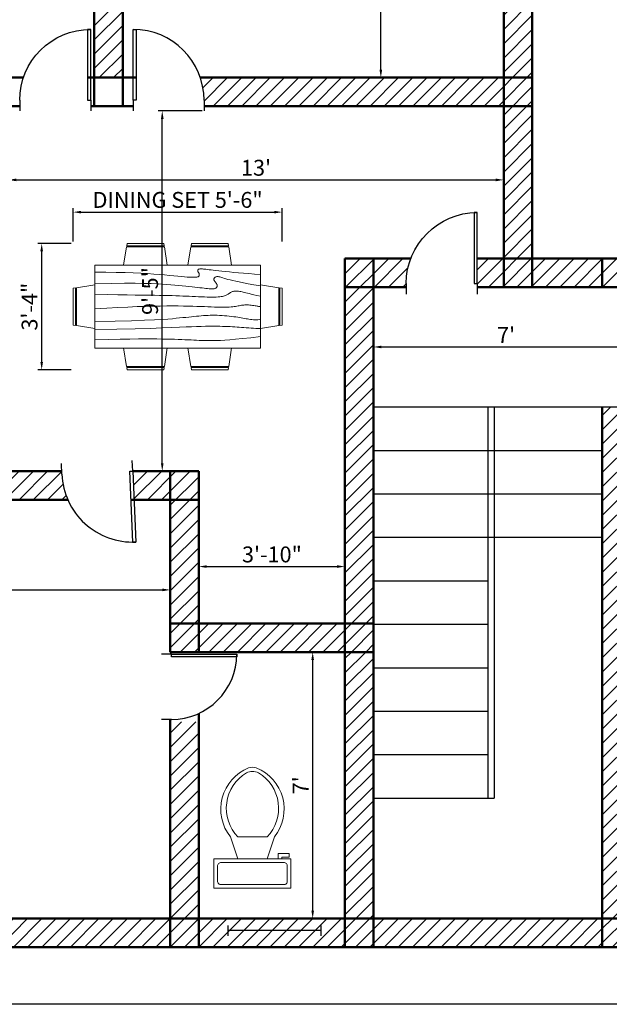
# Model space of a CAD drawing. Units: millimetres. Extents: x 2039 to 2694, y 890 to 1415.
# Tile 2 of 4: x 2216 to 2402, y 921 to 1232. Entities that reach past the tile are written whole.
import ezdxf

# ---------------------------------------------------------------- set-up
doc = ezdxf.new("R2010")
doc.units = ezdxf.units.MM
for name, color, linetype, lineweight in [('A-ANNO-DIMS', 80, 'Continuous', 18), ('A-FLOR-FIXT', 140, 'Continuous', 18), ('A-FLOR-STRS', 40, 'Continuous', 25), ('A-WALL-PATT', 6, 'Continuous', 13), ('doors', 10, 'Continuous', 25), ('furniture', 140, 'Continuous', 18), ('walls', 200, 'Continuous', 50), ('windows', 30, 'Continuous', 25)]:
    doc.layers.add(name, color=color, linetype=linetype, lineweight=lineweight)
doc.styles.get("Standard").update_dxf_attribs({"font": 'arial.ttf'})
doc.dimstyles.new('ISO-25', dxfattribs={"dimtxt": 5, "dimasz": 2.5, "dimexe": 1.25, "dimexo": 0.625, "dimtad": 1, "dimdec": 0, "dimlunit": 3, "dimtxsty": 'Standard', "dimcen": 2.5, "dimadec": 0, "dimazin": 0, "dimtfac": 1, "dimtdec": 0, "dimtmove": 0, "dimatfit": 3, "dimfxl": 1, "dimarcsym": 0})

# ---------------------------------------------------------------- blocks, each defined once
blk = doc.blocks.new('*U2')
for p, q in [((0, 0), (0, -6)), ((40, 0), (40, -6))]:
    blk.add_line(p, q)
blk.add_lwpolyline([(0, 0), (0, 40), (1.75, 40), (1.75, 0)], close=True)
blk.add_arc((0, 0), 40, 0, 90)
blk = doc.blocks.new('*U5')
for p, q in [((0, 4), (0, 0)), ((36, 4), (36, 0)), ((0, 2), (36, 2))]:
    blk.add_line(p, q)
blk = doc.blocks.new('Toilet - top')
for p, q in [((9.5, -6), (9.5, -2)), ((-8, -8.5), (-8, -8)), ((-7, -8), (-7, -9.5)), ((-4, -8), (-6, -14)), ((4, -8), (6, -14)), ((-10, -8.5), (-8, -8.5)), ((-10, -9.5), (-10, -8.5)), ((-7, -9.5), (-10, -9.5)), ((4, -14), (-4, -14))]:
    blk.add_line(p, q)
blk.add_lwpolyline([(10.5, -8), (10.5, 0), (-10.5, 0), (-10.5, -8)], close=True)
for points in [[(-9.5, -2), (-9.5, -6)], [(8.5, -1), (-8.5, -1)], [(-8.5, -7), (8.5, -7)]]:
    blk.add_lwpolyline(points)
for centre, radius, start, end in [((-8.62, -1.88), 0.884, 81.8699, 188.1301), ((8.62, -1.88), 0.884, 351.8699, 98.1301), ((-8.62, -6.12), 0.884, 171.8699, 278.1301), ((8.62, -6.12), 0.884, 261.8699, 8.1301), ((3.52, -21.58), 12.17, 141.4691, 247.9714), ((4.2, -21.82), 11.33, 136.3677, 238.9468), ((-3.52, -21.58), 12.17, 292.0284, 38.5307), ((-4.2, -21.82), 11.33, 301.053, 43.6321), ((0, -27.88), 4, 245.7318, 294.2682), ((0, -29), 4, 254.8605, 285.1395)]:
    blk.add_arc(centre, radius, start, end)
blk = doc.blocks.new('*D9')
at = {"layer": 'A-ANNO-DIMS', "color": 0, "lineweight": -2, "transparency": 16777216}
for p, q in [((2327.91, 1110.14), (2327.91, 1129.64)), ((2411.41, 1110.14), (2411.41, 1129.64)), ((2330.41, 1128.39), (2408.91, 1128.39))]:
    blk.add_line(p, q, dxfattribs=at)
at = {"layer": 'A-ANNO-DIMS', "color": 0, "transparency": 16777216}
for points in [[(2330.41, 1128.81), (2330.41, 1127.98), (2327.91, 1128.39)], [(2408.91, 1128.81), (2408.91, 1127.98), (2411.41, 1128.39)]]:
    blk.add_solid(points, dxfattribs=at)
at = {"layer": 'Defpoints', "color": 0, "transparency": 16777216}
for p in [(2411.41, 1128.39), (2327.91, 1109.51), (2411.41, 1109.51)]:
    blk.add_point(p, dxfattribs=at)
at = {"layer": 'A-ANNO-DIMS', "color": 0, "transparency": 16777216, "insert": (2369.66, 1131.52), "char_height": 5, "attachment_point": 5}
blk.add_mtext("7'", dxfattribs=at)
blk = doc.blocks.new('*D13')
at = {"layer": 'A-ANNO-DIMS', "color": 0, "lineweight": -2, "transparency": 16777216}
for p, q in [((2326.26, 1333.28), (2331.46, 1333.28)), ((2330.21, 1215.78), (2330.21, 1330.78)), ((2326.26, 1213.28), (2331.46, 1213.28))]:
    blk.add_line(p, q, dxfattribs=at)
at = {"layer": 'A-ANNO-DIMS', "color": 0, "transparency": 16777216}
for points in [[(2329.79, 1330.78), (2330.63, 1330.78), (2330.21, 1333.28)], [(2329.79, 1215.78), (2330.63, 1215.78), (2330.21, 1213.28)]]:
    blk.add_solid(points, dxfattribs=at)
at = {"layer": 'Defpoints', "color": 0, "transparency": 16777216}
for p in [(2325.64, 1333.28), (2330.21, 1333.28), (2325.64, 1213.28)]:
    blk.add_point(p, dxfattribs=at)
at = {"layer": 'A-ANNO-DIMS', "color": 0, "transparency": 16777216, "insert": (2327.03, 1273.28), "char_height": 5, "attachment_point": 5, "rotation": 90}
blk.add_mtext("10'", dxfattribs=at)
blk = doc.blocks.new('*D18')
at = {"layer": 'A-ANNO-DIMS', "color": 0, "lineweight": -2, "transparency": 16777216}
for p, q in [((2212.91, 1162.32), (2212.91, 1182.29)), ((2368.91, 1162.32), (2368.91, 1182.29)), ((2215.41, 1181.04), (2366.41, 1181.04))]:
    blk.add_line(p, q, dxfattribs=at)
at = {"layer": 'A-ANNO-DIMS', "color": 0, "transparency": 16777216}
for points in [[(2215.41, 1181.46), (2215.41, 1180.62), (2212.91, 1181.04)], [(2366.41, 1181.46), (2366.41, 1180.62), (2368.91, 1181.04)]]:
    blk.add_solid(points, dxfattribs=at)
at = {"layer": 'Defpoints', "color": 0, "transparency": 16777216}
for p in [(2368.91, 1181.04), (2212.91, 1161.69), (2368.91, 1161.69)]:
    blk.add_point(p, dxfattribs=at)
at = {"layer": 'A-ANNO-DIMS', "color": 0, "transparency": 16777216, "insert": (2290.91, 1184.22), "char_height": 5, "attachment_point": 5}
blk.add_mtext("13'", dxfattribs=at)
blk = doc.blocks.new('*D19')
at = {"layer": 'A-ANNO-DIMS', "color": 0, "lineweight": -2, "transparency": 16777216}
for p, q in [((2273.92, 1202.77), (2260.12, 1202.77)), ((2261.37, 1091.78), (2261.37, 1200.27)), ((2272.28, 1089.28), (2260.12, 1089.28))]:
    blk.add_line(p, q, dxfattribs=at)
at = {"layer": 'A-ANNO-DIMS', "color": 0, "transparency": 16777216}
for points in [[(2260.96, 1200.27), (2261.79, 1200.27), (2261.37, 1202.77)], [(2260.96, 1091.78), (2261.79, 1091.78), (2261.37, 1089.28)]]:
    blk.add_solid(points, dxfattribs=at)
at = {"layer": 'Defpoints', "color": 0, "transparency": 16777216}
for p in [(2261.37, 1202.77), (2274.54, 1202.77), (2272.91, 1089.28)]:
    blk.add_point(p, dxfattribs=at)
at = {"layer": 'A-ANNO-DIMS', "color": 0, "transparency": 16777216, "insert": (2258.19, 1146.02), "char_height": 5, "attachment_point": 5, "rotation": 90}
blk.add_mtext('9\'-5"', dxfattribs=at)
blk = doc.blocks.new('*D20')
at = {"layer": 'A-ANNO-DIMS', "color": 0, "lineweight": -2, "transparency": 16777216}
for p, q in [((2272.91, 1062.7), (2272.91, 1057.95)), ((2318.91, 1062.7), (2318.91, 1057.95)), ((2275.41, 1059.2), (2316.41, 1059.2))]:
    blk.add_line(p, q, dxfattribs=at)
at = {"layer": 'A-ANNO-DIMS', "color": 0, "transparency": 16777216}
for points in [[(2275.41, 1059.62), (2275.41, 1058.79), (2272.91, 1059.2)], [(2316.41, 1059.62), (2316.41, 1058.79), (2318.91, 1059.2)]]:
    blk.add_solid(points, dxfattribs=at)
at = {"layer": 'Defpoints', "color": 0, "transparency": 16777216}
for p in [(2272.91, 1063.32), (2318.91, 1063.32), (2318.91, 1059.2)]:
    blk.add_point(p, dxfattribs=at)
at = {"layer": 'A-ANNO-DIMS', "color": 0, "transparency": 16777216, "insert": (2295.91, 1062.38), "char_height": 5, "attachment_point": 5}
blk.add_mtext('3\'-10"', dxfattribs=at)
blk = doc.blocks.new('*D21')
at = {"layer": 'A-ANNO-DIMS', "color": 0, "lineweight": -2, "transparency": 16777216}
for p, q in [((2313.37, 1032.28), (2307.5, 1032.28)), ((2308.75, 950.78), (2308.75, 1029.78)), ((2313.37, 948.28), (2307.5, 948.28))]:
    blk.add_line(p, q, dxfattribs=at)
at = {"layer": 'A-ANNO-DIMS', "color": 0, "transparency": 16777216}
for points in [[(2308.33, 1029.78), (2309.16, 1029.78), (2308.75, 1032.28)], [(2308.33, 950.78), (2309.16, 950.78), (2308.75, 948.28)]]:
    blk.add_solid(points, dxfattribs=at)
at = {"layer": 'Defpoints', "color": 0, "transparency": 16777216}
for p in [(2308.75, 1032.28), (2314, 1032.28), (2314, 948.28)]:
    blk.add_point(p, dxfattribs=at)
at = {"layer": 'A-ANNO-DIMS', "color": 0, "transparency": 16777216, "insert": (2305.62, 990.28), "char_height": 5, "attachment_point": 5, "rotation": 90}
blk.add_mtext("7'", dxfattribs=at)
blk = doc.blocks.new('*D22')
at = {"layer": 'A-ANNO-DIMS', "color": 0, "lineweight": -2, "transparency": 16777216}
for p, q in [((2116.59, 1036.07), (2116.59, 1053.1)), ((2119.09, 1051.85), (2261.41, 1051.85)), ((2263.91, 1036.07), (2263.91, 1053.1))]:
    blk.add_line(p, q, dxfattribs=at)
at = {"layer": 'A-ANNO-DIMS', "color": 0, "transparency": 16777216}
for points in [[(2119.09, 1052.27), (2119.09, 1051.44), (2116.59, 1051.85)], [(2261.41, 1052.27), (2261.41, 1051.44), (2263.91, 1051.85)]]:
    blk.add_solid(points, dxfattribs=at)
at = {"layer": 'Defpoints', "color": 0, "transparency": 16777216}
for p in [(2263.91, 1051.85), (2116.59, 1035.45), (2263.91, 1035.45)]:
    blk.add_point(p, dxfattribs=at)
at = {"layer": 'A-ANNO-DIMS', "color": 0, "transparency": 16777216, "insert": (2190.25, 1055.03), "char_height": 5, "attachment_point": 5}
blk.add_mtext('12\'-3"', dxfattribs=at)
blk = doc.blocks.new('Dining Set - 36 x 72 in.')
for p, q in [((-22.2343, 26.00059), (-23.4847, 17.99762)), ((-22.2304, 26), (-5.7608, 26)), ((-22, 27.5), (-22.1562, 26.50042)), ((-5.8416, 26.5), (-22.1534, 26.5)), ((-22, 27.5), (-6, 27.5)), ((-5.8437, 26.49966), (-6, 27.5)), ((-4.5152, 17.99762), (-5.7655, 25.99926)), ((5.7657, 26.00059), (4.5153, 17.99762)), ((5.7696, 26), (22.2392, 26)), ((6, 27.5), (5.8438, 26.50042)), ((22.1584, 26.5), (5.8466, 26.5)), ((6, 27.5), (22, 27.5)), ((22.1563, 26.49966), (22, 27.5)), ((23.4848, 17.99762), (22.2345, 25.99926)), ((36, 18), (-36, 18)), ((-36, 18), (-36, -18)), ((36, -18), (36, 18)), ((-44.0006, 8.23428), (-35.9976, 9.48474)), ((44.0006, 8.23428), (35.9976, 9.48474)), ((-45.5, 8), (-44.5004, 8.15617)), ((-45.5, 8), (-45.5, -8)), ((-44.5, -8.15843), (-44.5, 8.15338)), ((-44, 8.23041), (-44, -8.23915)), ((44, 8.23041), (44, -8.23915)), ((44.5, -8.15843), (44.5, 8.15338)), ((45.5, 8), (44.5005, 8.15617)), ((45.5, 8), (45.5, -8)), ((-44.4997, -8.15631), (-45.5, -8)), ((-35.9976, -9.48476), (-43.9993, -8.2345)), ((35.9976, -9.48476), (43.9993, -8.2345)), ((44.4997, -8.15631), (45.5, -8)), ((-36, -18), (36, -18)), ((-22.2343, -26.0006), (-23.4847, -17.99762)), ((-4.5152, -17.99762), (-5.7655, -25.99928)), ((5.7657, -26.0006), (4.5153, -17.99762)), ((23.4848, -17.99762), (22.2345, -25.99928)), ((-22.2304, -26), (-5.7608, -26)), ((-22, -27.5), (-22.1562, -26.50044)), ((-5.8416, -26.5), (-22.1534, -26.5)), ((-22, -27.5), (-6, -27.5)), ((-5.8437, -26.49967), (-6, -27.5)), ((5.7696, -26), (22.2392, -26)), ((6, -27.5), (5.8438, -26.50044)), ((22.1584, -26.5), (5.8466, -26.5)), ((6, -27.5), (22, -27.5)), ((22.1563, -26.49967), (22, -27.5))]:
    blk.add_line(p, q)
for points in [[(-36, 15), (-31.1772, 14.97754), (-26.8079, 14.91406), (-22.8538, 14.81543), (-19.276, 14.6875), (-16.0362, 14.53613), (-13.0957, 14.36718), (-10.4159, 14.18652), (-7.9583, 14), (-5.6904, 13.81315), (-3.6035, 13.63021), (-1.6954, 13.45508), (0.0365, 13.29166), (1.5945, 13.14388), (2.9811, 13.01562), (4.1988, 12.9108), (5.25, 12.83333), (6.1393, 12.78613), (6.8802, 12.76823), (7.4883, 12.77767), (7.9792, 12.8125), (8.3685, 12.87077), (8.6719, 12.95052), (8.9049, 13.0498), (9.0833, 13.16666), (9.2205, 13.29899), (9.3216, 13.44401), (9.3895, 13.59879), (9.4271, 13.76041), (9.4373, 13.92594), (9.4232, 14.09245), (9.3875, 14.257), (9.3333, 14.41666), (9.2638, 14.56917), (9.1836, 14.71484), (9.0975, 14.85465), (9.0104, 14.98958), (8.9272, 15.1206), (8.8529, 15.2487), (8.7922, 15.37483), (8.75, 15.5), (8.7305, 15.62467), (8.7344, 15.74739), (8.7617, 15.86621), (8.8125, 15.97916), (8.8867, 16.08431), (8.9844, 16.17968), (9.1055, 16.26334), (9.25, 16.33333), (9.4189, 16.38802), (9.6172, 16.42708), (9.8506, 16.45052), (10.125, 16.45833), (10.4463, 16.45052), (10.8203, 16.42708), (11.2529, 16.38802), (11.75, 16.33333), (12.3184, 16.26318), (12.9694, 16.17838), (13.7151, 16.07991), (14.5677, 15.96875), (15.5395, 15.84586), (16.6426, 15.71224), (17.8893, 15.56884), (19.2917, 15.41666), (20.859, 15.25667), (22.5879, 15.08984), (24.4721, 14.91715), (26.5052, 14.73958), (28.6809, 14.5581), (30.9929, 14.3737), (33.4347, 14.18733), (36, 14)], [(-36, 10), (-28.9766, 10.14274), (-23.1725, 10.20442), (-18.4241, 10.19775), (-14.5677, 10.13541), (-11.4399, 10.03011), (-8.877, 9.89453), (-6.7154, 9.74137), (-4.7917, 9.58333), (-2.9698, 9.43082), (-1.2246, 9.28515), (0.4415, 9.14534), (2.026, 9.01041), (3.5266, 8.87939), (4.9408, 8.7513), (6.266, 8.62516), (7.5, 8.5), (8.6411, 8.37549), (9.6914, 8.2539), (10.6538, 8.13818), (11.5312, 8.03125), (12.3267, 7.93603), (13.043, 7.85547), (13.6831, 7.79248), (14.25, 7.75), (14.7471, 7.7303), (15.1797, 7.73307), (15.5537, 7.75732), (15.875, 7.80208), (16.1494, 7.86637), (16.3828, 7.94922), (16.5811, 8.04964), (16.75, 8.16666), (16.8944, 8.29915), (17.0143, 8.44531), (17.1089, 8.60319), (17.1771, 8.77083), (17.218, 8.94629), (17.2305, 9.1276), (17.2137, 9.31282), (17.1667, 9.5), (17.0895, 9.6875), (16.987, 9.875), (16.8649, 10.0625), (16.7292, 10.25), (16.5856, 10.4375), (16.4401, 10.625), (16.2985, 10.8125), (16.1667, 11), (16.05, 11.18733), (15.9518, 11.3737), (15.8752, 11.5581), (15.8229, 11.73958), (15.798, 11.91715), (15.8034, 12.08984), (15.842, 12.25667), (15.9167, 12.41666), (16.0295, 12.56836), (16.1784, 12.70833), (16.3605, 12.83268), (16.5729, 12.9375), (16.8127, 13.01888), (17.0768, 13.07291), (17.3625, 13.0957), (17.6667, 13.08333), (17.9894, 13.03312), (18.3418, 12.94726), (18.7382, 12.82918), (19.1927, 12.68229), (19.7195, 12.51001), (20.3327, 12.31575), (21.0465, 12.10294), (21.875, 11.875), (22.8357, 11.63354), (23.959, 11.37304), (25.2786, 11.08618), (26.8282, 10.76562), (28.6414, 10.40405), (30.752, 9.99414), (33.1936, 9.52856), (36, 9)], [(-36, 5.5), (-30.7157, 5.3348), (-26.069, 5.20963), (-21.9946, 5.11767), (-18.4271, 5.05208), (-15.3009, 5.00602), (-12.5508, 4.97265), (-10.1112, 4.94515), (-7.9167, 4.91666), (-5.909, 4.88167), (-4.0586, 4.83984), (-2.3429, 4.79215), (-0.7396, 4.73958), (0.7739, 4.6831), (2.22, 4.6237), (3.6213, 4.56233), (5, 4.5), (6.373, 4.43782), (7.7344, 4.3776), (9.0723, 4.32129), (10.375, 4.27083), (11.6309, 4.22819), (12.8281, 4.19531), (13.9551, 4.17415), (15, 4.16666), (15.954, 4.17448), (16.819, 4.19791), (17.6001, 4.23698), (18.3021, 4.29166), (18.9299, 4.36198), (19.4883, 4.44791), (19.9823, 4.54948), (20.4167, 4.66666), (20.7969, 4.79899), (21.1302, 4.94401), (21.4245, 5.09879), (21.6875, 5.26041), (21.9271, 5.42594), (22.1511, 5.59245), (22.3672, 5.757), (22.5834, 5.91666), (22.8065, 6.06868), (23.0404, 6.21093), (23.2879, 6.34147), (23.5521, 6.45833), (23.8358, 6.55957), (24.142, 6.64323), (24.4735, 6.70735), (24.8334, 6.75), (25.2235, 6.76969), (25.642, 6.76692), (26.0858, 6.74267), (26.5521, 6.69791), (27.0379, 6.63362), (27.5404, 6.55078), (28.0565, 6.45036), (28.5834, 6.33333), (29.1242, 6.19987), (29.7071, 6.04687), (30.3661, 5.87044), (31.1354, 5.66666), (32.0493, 5.43164), (33.142, 5.16146), (34.4475, 4.85221), (36, 4.5)], [(-36, -1), (-30.7915, -0.6591), (-26.0195, -0.38216), (-21.6519, -0.16284), (-17.6563, 0.00521), (-14.0005, 0.12833), (-10.6523, 0.21289), (-7.5796, 0.26522), (-4.75, 0.29166), (-2.134, 0.29793), (0.2878, 0.28711), (2.5317, 0.26163), (4.6146, 0.22396), (6.5529, 0.17651), (8.3633, 0.12174), (10.0623, 0.06209), (11.6667, 0), (13.1899, -0.06201), (14.6341, -0.1211), (15.9982, -0.17432), (17.2813, -0.21875), (18.4823, -0.25147), (19.6003, -0.26953), (20.6343, -0.27002), (21.5834, -0.25), (22.4481, -0.20768), (23.2357, -0.14584), (23.9549, -0.06836), (24.6146, 0.02083), (25.2235, 0.11784), (25.7904, 0.21875), (26.3241, 0.31966), (26.8334, 0.41666), (27.3265, 0.50618), (27.8099, 0.58593), (28.2894, 0.65397), (28.7709, 0.70833), (29.2601, 0.74707), (29.763, 0.76823), (30.2855, 0.76985), (30.8334, 0.75), (31.4088, 0.70784), (31.9994, 0.64713), (32.589, 0.57275), (33.1615, 0.48958), (33.7008, 0.4025), (34.1908, 0.3164), (34.6153, 0.23616), (34.9584, 0.16666), (35.2099, 0.11165), (35.3848, 0.07031), (35.504, 0.04069), (35.5886, 0.02083), (35.6594, 0.00879), (35.7377, 0.0026), (35.8442, 0.00032), (36, 0)], [(-36, -6.5), (-27.1843, -6.31267), (-20.084, -6.1263), (-14.469, -5.9419), (-10.1094, -5.76042), (-6.7752, -5.58285), (-4.2363, -5.41016), (-2.2629, -5.24333), (-0.625, -5.08334), (0.8708, -4.93099), (2.2715, -4.78646), (3.5872, -4.64974), (4.8281, -4.52084), (6.0046, -4.39974), (7.127, -4.28646), (8.2053, -4.18099), (9.25, -4.08334), (10.2705, -3.99382), (11.2734, -3.91407), (12.2647, -3.84603), (13.25, -3.79167), (14.2354, -3.75293), (15.2266, -3.73177), (16.2295, -3.73015), (17.25, -3.75), (18.2912, -3.79248), (19.3451, -3.85547), (20.4009, -3.93604), (21.4479, -4.03125), (22.4754, -4.13819), (23.4727, -4.25391), (24.4289, -4.37549), (25.3334, -4.5), (26.1785, -4.62492), (26.9694, -4.74935), (27.7145, -4.87281), (28.4219, -4.99479), (29.1, -5.11483), (29.7572, -5.23242), (30.4016, -5.34709), (31.0417, -5.45834), (31.6837, -5.56437), (32.3262, -5.65821), (32.9658, -5.73153), (33.599, -5.77604), (34.2224, -5.78345), (34.8327, -5.74545), (35.4264, -5.65373), (36, -5.5)], [(-36, -10), (-26.4022, -9.81299), (-18.4675, -9.62891), (-11.9839, -9.45069), (-6.7396, -9.28125), (-2.5226, -9.12354), (0.8789, -8.98047), (3.6769, -8.85498), (6.0833, -8.75), (8.2767, -8.66765), (10.3021, -8.60677), (12.1712, -8.56543), (13.8958, -8.54167), (15.4876, -8.53353), (16.9583, -8.53907), (18.3197, -8.55632), (19.5834, -8.58334), (20.7616, -8.61841), (21.8685, -8.66081), (22.9188, -8.71004), (23.9271, -8.76563), (24.9081, -8.82707), (25.8763, -8.89388), (26.8465, -8.96558), (27.8334, -9.04167), (28.8474, -9.12118), (29.8828, -9.20117), (30.93, -9.27824), (31.9792, -9.34896), (33.0205, -9.40991), (34.0443, -9.45768), (35.0407, -9.48885), (36, -9.5)], [(-36, -14.5), (-30.0881, -14.33513), (-25.0332, -14.21224), (-20.7312, -14.12647), (-17.0781, -14.07292), (-13.97, -14.04671), (-11.3027, -14.04297), (-8.9724, -14.05681), (-6.875, -14.08334), (-4.9224, -14.11833), (-3.0905, -14.16016), (-1.3709, -14.20785), (0.2448, -14.26042), (1.7647, -14.3169), (3.1973, -14.3763), (4.5507, -14.43767), (5.8333, -14.5), (7.0554, -14.5621), (8.235, -14.62175), (9.3922, -14.67652), (10.5469, -14.72396), (11.7192, -14.76164), (12.929, -14.78711), (14.1965, -14.79794), (15.5417, -14.79167), (16.9933, -14.76424), (18.6152, -14.70508), (20.4804, -14.60197), (22.6615, -14.44271), (25.2312, -14.21509), (28.2624, -13.9069), (31.8277, -13.50594), (36, -13)]]:
    blk.add_lwpolyline(points)
blk = doc.blocks.new('*D33')
at = {"layer": 'A-ANNO-DIMS', "color": 0, "lineweight": -2, "transparency": 16777216}
for p, q in [((2233.28, 1161.63), (2233.28, 1172.13)), ((2235.78, 1170.88), (2296.64, 1170.88)), ((2299.14, 1161.63), (2299.14, 1172.13))]:
    blk.add_line(p, q, dxfattribs=at)
at = {"layer": 'A-ANNO-DIMS', "color": 0, "transparency": 16777216}
for points in [[(2235.78, 1171.3), (2235.78, 1170.47), (2233.28, 1170.88)], [(2296.64, 1171.3), (2296.64, 1170.47), (2299.14, 1170.88)]]:
    blk.add_solid(points, dxfattribs=at)
at = {"layer": 'Defpoints', "color": 0, "transparency": 16777216}
for p in [(2299.14, 1170.88), (2233.28, 1161), (2299.14, 1161)]:
    blk.add_point(p, dxfattribs=at)
at = {"layer": 'A-ANNO-DIMS', "color": 0, "transparency": 16777216, "insert": (2266.21, 1174.09), "char_height": 5, "attachment_point": 5}
blk.add_mtext('DINING SET 5\'-6"', dxfattribs=at)
blk = doc.blocks.new('*D34')
at = {"layer": 'A-ANNO-DIMS', "color": 0, "lineweight": -2, "transparency": 16777216}
for p, q in [((2232.65, 1161), (2222.15, 1161)), ((2223.4, 1123.7), (2223.4, 1158.5)), ((2232.65, 1121.2), (2222.15, 1121.2))]:
    blk.add_line(p, q, dxfattribs=at)
at = {"layer": 'A-ANNO-DIMS', "color": 0, "transparency": 16777216}
for points in [[(2222.98, 1158.5), (2223.82, 1158.5), (2223.4, 1161)], [(2222.98, 1123.7), (2223.82, 1123.7), (2223.4, 1121.2)]]:
    blk.add_solid(points, dxfattribs=at)
at = {"layer": 'Defpoints', "color": 0, "transparency": 16777216}
for p in [(2223.4, 1161), (2233.28, 1161), (2233.28, 1121.2)]:
    blk.add_point(p, dxfattribs=at)
at = {"layer": 'A-ANNO-DIMS', "color": 0, "transparency": 16777216, "insert": (2220.22, 1141.1), "char_height": 5, "attachment_point": 5, "rotation": 90}
blk.add_mtext('3\'-4"', dxfattribs=at)
blk = doc.blocks.new('*D39')
at = {"layer": 'A-ANNO-DIMS', "color": 0, "lineweight": -2, "transparency": 16777216}
for p, q in [((2408.28, 939.28), (2043.96, 939.28)), ((2045.21, 923.78), (2045.21, 936.78)), ((2408.28, 921.28), (2043.96, 921.28))]:
    blk.add_line(p, q, dxfattribs=at)
at = {"layer": 'A-ANNO-DIMS', "color": 0, "transparency": 16777216}
for points in [[(2044.79, 936.78), (2045.62, 936.78), (2045.21, 939.28)], [(2044.79, 923.78), (2045.62, 923.78), (2045.21, 921.28)]]:
    blk.add_solid(points, dxfattribs=at)
at = {"layer": 'Defpoints', "color": 0, "transparency": 16777216}
for p in [(2045.21, 939.28), (2408.91, 939.28), (2408.91, 921.28)]:
    blk.add_point(p, dxfattribs=at)
at = {"layer": 'A-ANNO-DIMS', "color": 0, "transparency": 16777216, "insert": (2042.03, 930.28), "char_height": 5, "attachment_point": 5, "rotation": 90}
blk.add_mtext('1\'-6"', dxfattribs=at)

msp = doc.modelspace()

# ---------------------------------------------------------------- hatches: boundary and pattern name
at = {"layer": 'A-WALL-PATT'}
h = msp.add_hatch(dxfattribs=at)
h.set_pattern_fill('ANSI31', color=256)
h.paths.add_polyline_path([(2119.91, 1333.28), (2110.91, 1333.28), (2110.91, 1213.28), (2119.91, 1213.28)])
h.paths.add_polyline_path([(2119.91, 1342.28), (2110.91, 1342.28), (2110.91, 1333.28), (2119.91, 1333.28)])
h.paths.add_polyline_path([(2239.91, 1342.28), (2119.91, 1342.28), (2119.91, 1333.28), (2239.91, 1333.28)])
h.paths.add_polyline_path([(2368.91, 1342.28), (2248.91, 1342.28), (2248.91, 1333.28), (2368.91, 1333.28)])
h.paths.add_polyline_path([(2248.91, 1342.28), (2239.91, 1342.28), (2239.91, 1333.28), (2248.91, 1333.28)])
h.paths.add_polyline_path([(2248.91, 1333.28), (2239.91, 1333.28), (2239.91, 1213.28), (2248.91, 1213.28)])
h.paths.add_polyline_path([(2203.91, 1213.28), (2119.91, 1213.28), (2119.91, 1204.28), (2203.91, 1204.28)])
h.paths.add_polyline_path([(2119.91, 1204.28), (2110.91, 1204.28), (2110.91, 1156.28), (2119.91, 1156.28)])
h.paths.add_polyline_path([(2119.91, 1213.28), (2110.91, 1213.28), (2110.91, 1204.28), (2119.91, 1204.28)])
h.paths.add_polyline_path([(2212.91, 1213.28), (2203.91, 1213.28), (2203.91, 1204.28), (2212.91, 1204.28)])
h.paths.add_polyline_path([(2368.91, 1213.28), (2273.37, 1213.28, -0.081603), (2274.54, 1206.12), (2274.54, 1204.28), (2368.91, 1204.28)])
h.paths.add_polyline_path([(2377.91, 1333.28), (2368.91, 1333.28), (2368.91, 1213.28), (2377.91, 1213.28)])
h.paths.add_polyline_path([(2617.91, 1342.28), (2377.91, 1342.28), (2377.91, 1333.28), (2617.91, 1333.28)])
h.paths.add_polyline_path([(2377.91, 1342.28), (2368.91, 1342.28), (2368.91, 1333.28), (2377.91, 1333.28)])
h.paths.add_polyline_path([(2626.91, 1333.28), (2617.91, 1333.28), (2617.91, 948.28), (2626.91, 948.28)])
h.paths.add_polyline_path([(2377.91, 1204.28), (2368.91, 1204.28), (2368.91, 1156.28), (2377.91, 1156.28)])
h.paths.add_polyline_path([(2377.91, 1156.28), (2368.91, 1156.28), (2368.91, 1147.28), (2377.91, 1147.28)])
h.paths.add_polyline_path([(2377.91, 1213.28), (2368.91, 1213.28), (2368.91, 1204.28), (2377.91, 1204.28)])
h.paths.add_polyline_path([(2368.91, 1156.28), (2360.56, 1156.28), (2360.56, 1148.39), (2360.56, 1147.28), (2368.91, 1147.28)])
h.paths.add_polyline_path([(2399.91, 1156.28), (2377.91, 1156.28), (2377.91, 1147.28), (2399.91, 1147.28)])
h.paths.add_polyline_path([(2408.91, 1156.28), (2399.91, 1156.28), (2399.91, 1147.28), (2408.91, 1147.28)])
h.paths.add_polyline_path([(2339.63, 1156.28), (2327.91, 1156.28), (2327.91, 1147.28), (2338.19, 1147.28), (2338.19, 1148.39, -0.090365)])
h.paths.add_polyline_path([(2327.91, 1156.28), (2318.91, 1156.28), (2318.91, 1147.28), (2327.91, 1147.28)])
h.paths.add_polyline_path([(2327.91, 1147.28), (2318.91, 1147.28), (2318.91, 1041.28), (2327.91, 1041.28)])
h.paths.add_polyline_path([(2408.91, 1109.51), (2399.91, 1109.51), (2399.91, 948.28), (2408.91, 948.28)])
h.paths.add_polyline_path([(2272.91, 1080.28), (2263.91, 1080.28), (2263.91, 1041.28), (2272.91, 1041.28)])
h.paths.add_polyline_path([(2272.91, 1089.28), (2263.91, 1089.28), (2263.91, 1080.28), (2272.91, 1080.28)])
h.paths.add_polyline_path([(2263.91, 1089.28), (2252.09, 1089.28), (2252.48, 1080.28), (2263.91, 1080.28)])
h.paths.add_polyline_path([(2229.75, 1088.3), (2229.7, 1089.28), (2212.91, 1089.28), (2212.91, 1080.28), (2231.62, 1080.28, -0.092884)])
h.paths.add_polyline_path([(2212.91, 1124.18), (2211.56, 1124.21, -0.10492), (2203.91, 1126.01), (2203.91, 1089.28), (2212.91, 1089.28)])
h.paths.add_polyline_path([(2212.91, 1089.28), (2203.91, 1089.28), (2203.91, 1080.28), (2212.91, 1080.28)])
h.paths.add_polyline_path([(2203.91, 1089.28), (2119.91, 1089.28), (2119.91, 1080.28), (2203.91, 1080.28)])
h.paths.add_polyline_path([(2119.91, 1147.28), (2110.91, 1147.28), (2110.91, 1089.28), (2119.91, 1089.28)])
h.paths.add_polyline_path([(2119.91, 1156.28), (2110.91, 1156.28), (2110.91, 1147.28), (2119.91, 1147.28)])
h.paths.add_polyline_path([(2203.91, 1156.28), (2119.91, 1156.28), (2119.91, 1147.28), (2136.91, 1147.28), (2203.91, 1147.28)])
h.paths.add_polyline_path([(2119.91, 1080.28), (2110.91, 1080.28), (2110.91, 948.28), (2119.91, 948.28)])
h.paths.add_polyline_path([(2119.91, 1089.28), (2110.91, 1089.28), (2110.91, 1080.28), (2119.91, 1080.28)])
h.paths.add_polyline_path([(2119.91, 948.28), (2110.91, 948.28), (2110.91, 939.28), (2119.91, 939.28)])
h.paths.add_polyline_path([(2263.91, 948.28), (2119.91, 948.28), (2119.91, 939.28), (2263.91, 939.28)])
h.paths.add_polyline_path([(2318.91, 948.28), (2272.91, 948.28), (2272.91, 939.28), (2318.91, 939.28)])
h.paths.add_polyline_path([(2272.91, 948.28), (2263.91, 948.28), (2263.91, 939.28), (2272.91, 939.28)])
h.paths.add_polyline_path([(2272.91, 1041.28), (2263.91, 1041.28), (2263.91, 1032.28), (2272.91, 1032.28)])
h.paths.add_polyline_path([(2327.91, 1032.28), (2318.91, 1032.28), (2318.91, 948.28), (2327.91, 948.28)])
h.paths.add_polyline_path([(2399.91, 948.28), (2327.91, 948.28), (2327.91, 939.28), (2399.91, 939.28)])
h.paths.add_polyline_path([(2327.91, 948.28), (2318.91, 948.28), (2318.91, 939.28), (2327.91, 939.28)])
h.paths.add_polyline_path([(2408.91, 948.28), (2399.91, 948.28), (2399.91, 939.28), (2408.91, 939.28)])
h.paths.add_polyline_path([(2617.91, 948.28), (2408.91, 948.28), (2408.91, 939.28), (2617.91, 939.28)])
h.paths.add_polyline_path([(2626.91, 948.28), (2617.91, 948.28), (2617.91, 939.28), (2626.91, 939.28)])
h.paths.add_polyline_path([(2132.32, 1149.06), (2159.44, 1149.06), (2159.44, 1167.69), (2132.32, 1167.69)], flags=9)
h = msp.add_hatch(dxfattribs=at)
h.set_pattern_fill('ANSI31', color=256)
h.paths.add_polyline_path([(2272.91, 999.96), (2263.91, 999.96), (2263.91, 948.28), (2272.91, 948.28)])
h.paths.add_polyline_path([(2318.91, 1041.28), (2272.91, 1041.28), (2272.91, 1032.28), (2318.91, 1032.28)])
h.paths.add_polyline_path([(2327.91, 1041.28), (2318.91, 1041.28), (2318.91, 1032.28), (2327.91, 1032.28)])
h = msp.add_hatch(dxfattribs=at)
h.set_pattern_fill('ANSI31', color=256)
h.paths.add_polyline_path([(2272.91, 1010.23), (2263.91, 1010.23), (2263.91, 999.96), (2263.91, 948.28), (2272.91, 948.28), (2272.91, 999.96)])

# ---------------------------------------------------------------- linework, layer by layer
at = {"layer": 'A-FLOR-STRS'}
for p, q in [((2327.91, 1109.51), (2418.41, 1109.51)), ((2363.91, 1109.51), (2363.91, 986.26)), ((2365.91, 1109.51), (2365.91, 986.26)), ((2327.91, 1095.82), (2399.91, 1095.82)), ((2327.91, 1082.12), (2399.91, 1082.12)), ((2327.91, 1068.43), (2399.91, 1068.43)), ((2327.91, 1054.73), (2363.91, 1054.73)), ((2327.91, 1041.04), (2363.91, 1041.04)), ((2327.91, 1027.34), (2363.91, 1027.34)), ((2327.91, 1013.65), (2363.91, 1013.65)), ((2327.91, 999.95), (2363.91, 999.95)), ((2327.91, 986.26), (2365.91, 986.26))]:
    msp.add_line(p, q, dxfattribs=at)
at = {"layer": 'walls'}
for p, q in [((2239.91, 1342.28), (2239.91, 1204.28)), ((2248.91, 1342.28), (2248.91, 1204.28)), ((2368.91, 1342.28), (2368.91, 1147.28)), ((2377.91, 1342.28), (2377.91, 1147.28)), ((2110.91, 1213.28), (2217.66, 1213.28)), ((2237.86, 1213.28), (2253.16, 1213.28)), ((2273.37, 1213.28), (2377.91, 1213.28)), ((2110.91, 1204.28), (2216.48, 1204.28)), ((2238.84, 1204.28), (2252.18, 1204.28)), ((2274.54, 1204.28), (2377.91, 1204.28)), ((2318.91, 1156.28), (2318.91, 939.28)), ((2318.91, 1156.28), (2339.63, 1156.28)), ((2327.91, 1156.28), (2327.91, 939.28)), ((2360.56, 1156.28), (2408.91, 1156.28)), ((2399.91, 1156.28), (2399.91, 1147.28)), ((2318.91, 1147.28), (2338.19, 1147.28)), ((2360.56, 1147.28), (2418.41, 1147.28)), ((2399.91, 1109.51), (2399.91, 939.28)), ((2110.91, 1089.28), (2229.7, 1089.28)), ((2252.09, 1089.28), (2272.91, 1089.28)), ((2263.91, 1089.28), (2263.91, 1032.28)), ((2272.91, 1089.28), (2272.91, 1032.28)), ((2110.91, 1080.28), (2231.62, 1080.28)), ((2251.5, 1080.28), (2272.91, 1080.28)), ((2263.91, 1041.28), (2327.91, 1041.28)), ((2263.91, 1032.28), (2327.91, 1032.28)), ((2272.91, 1012.93), (2272.91, 999.96)), ((2263.91, 999.96), (2263.91, 1011.02)), ((2263.91, 999.96), (2263.91, 939.28)), ((2272.91, 999.96), (2272.91, 939.28)), ((2110.91, 948.28), (2626.91, 948.28)), ((2110.91, 939.28), (2626.91, 939.28))]:
    msp.add_line(p, q, dxfattribs=at)

# ---------------------------------------------------------------- block references
at = {"layer": 'A-FLOR-FIXT', "xscale": 1.154546597564434, "yscale": 1.154546597564434, "zscale": 1.154546597564434, "rotation": 179.999995176937}
msp.add_blockref('Toilet - top', (2289.78, 957.85), dxfattribs=at)
at = {"layer": 'doors', "yscale": 0.559018698302236, "zscale": 0.559018698302236}
for p, xscale in [((2238.84, 1206.12), -0.559018698302236), ((2252.18, 1206.12), 0.559018698302236), ((2360.56, 1148.39), -0.559018698302236)]:
    msp.add_blockref('*U2', p, dxfattribs=dict(at, xscale=xscale))
at = {"layer": 'doors'}
for p, xscale, yscale, zscale, rotation in [((2252.09, 1089.28), 0.559018698302236, 0.559018698302236, 0.559018698302236, 182.5074966702692), ((2264.24, 1031.64), 0.5154017243196501, 0.5154017243196501, 0.5154017243196501, 270)]:
    msp.add_blockref('*U2', p, dxfattribs=dict(at, xscale=xscale, yscale=yscale, zscale=zscale, rotation=rotation))
at = {"layer": 'furniture', "xscale": 0.7237386186581148, "yscale": 0.7237386186581148, "zscale": 0.7237386186581148}
msp.add_blockref('Dining Set - 36 x 72 in.', (2266.21, 1141.1), dxfattribs=at)
at = {"layer": 'windows', "xscale": 0.8142679173318405, "yscale": 0.8142679173318405, "zscale": 0.8142679173318405, "rotation": 180}
msp.add_blockref('*U5', (2311.41, 946.12), dxfattribs=at)

# ---------------------------------------------------------------- dimensions: what is measured, and where the dimension line sits
at = {"layer": 'A-ANNO-DIMS'}
for base, p1, p2, override, picture, middle in [((2330.21, 1333.28), (2325.64, 1213.28), (2325.64, 1333.28), {"dimclrd": 0, "dimclre": 0, "dimclrt": 0}, '*D13', (2327.03, 1273.28)), ((2261.37, 1202.77), (2272.91, 1089.28), (2274.54, 1202.77), {"dimclrd": 0, "dimclre": 0, "dimclrt": 0}, '*D19', (2258.19, 1146.02)), ((2223.4, 1161), (2233.28, 1121.2), (2233.28, 1161), {"dimdec": 1, "dimlfac": 1, "dimrnd": 0, "dimzin": 1, "dimdsep": 46, "dimlunit": 4, "dimfrac": 2}, '*D34', (2220.22, 1141.1)), ((2308.75, 1032.28), (2314, 948.28), (2314, 1032.28), {"dimclrd": 0, "dimclre": 0, "dimclrt": 0}, '*D21', (2305.62, 990.28)), ((2045.21, 939.28), (2408.91, 921.28), (2408.91, 939.28), {"dimdec": 1, "dimlfac": 1, "dimrnd": 0, "dimzin": 1, "dimdsep": 46, "dimlunit": 4, "dimfrac": 2}, '*D39', (2042.03, 930.28))]:
    dim = msp.add_linear_dim(base=base, p1=p1, p2=p2, angle=90, dimstyle='ISO-25', override=override, dxfattribs=at)
    dim.commit()
    dim.dimension.update_dxf_attribs({"geometry": picture, "text_midpoint": middle})
for base, p1, p2, picture, middle in [((2368.91, 1181.04), (2212.91, 1161.69), (2368.91, 1161.69), '*D18', (2290.91, 1184.22)), ((2411.40500058, 1128.39421206), (2327.90500058, 1109.51214927), (2411.40500058, 1109.51214927), '*D9', (2369.65500058, 1131.51921206)), ((2318.91, 1059.2), (2272.91, 1063.32), (2318.91, 1063.32), '*D20', (2295.91, 1062.38)), ((2263.91, 1051.85), (2116.59, 1035.45), (2263.91, 1035.45), '*D22', (2190.25, 1055.03))]:
    dim = msp.add_linear_dim(base=base, p1=p1, p2=p2, dimstyle='ISO-25', override={"dimclrd": 0, "dimclre": 0, "dimclrt": 0}, dxfattribs=at)
    dim.commit()
    dim.dimension.update_dxf_attribs({"geometry": picture, "text_midpoint": middle})
dim = msp.add_linear_dim(base=(2299.14, 1170.88), p1=(2233.28, 1161), p2=(2299.14, 1161), text='DINING SET <>', dimstyle='ISO-25', override={"dimdec": 1, "dimlfac": 1, "dimrnd": 0, "dimzin": 1, "dimdsep": 46, "dimlunit": 4, "dimfrac": 2}, dxfattribs=at)
dim.commit()
dim.dimension.update_dxf_attribs({"geometry": '*D33', "text_midpoint": (2266.21, 1174.09)})

doc.saveas('drawing.dxf')
